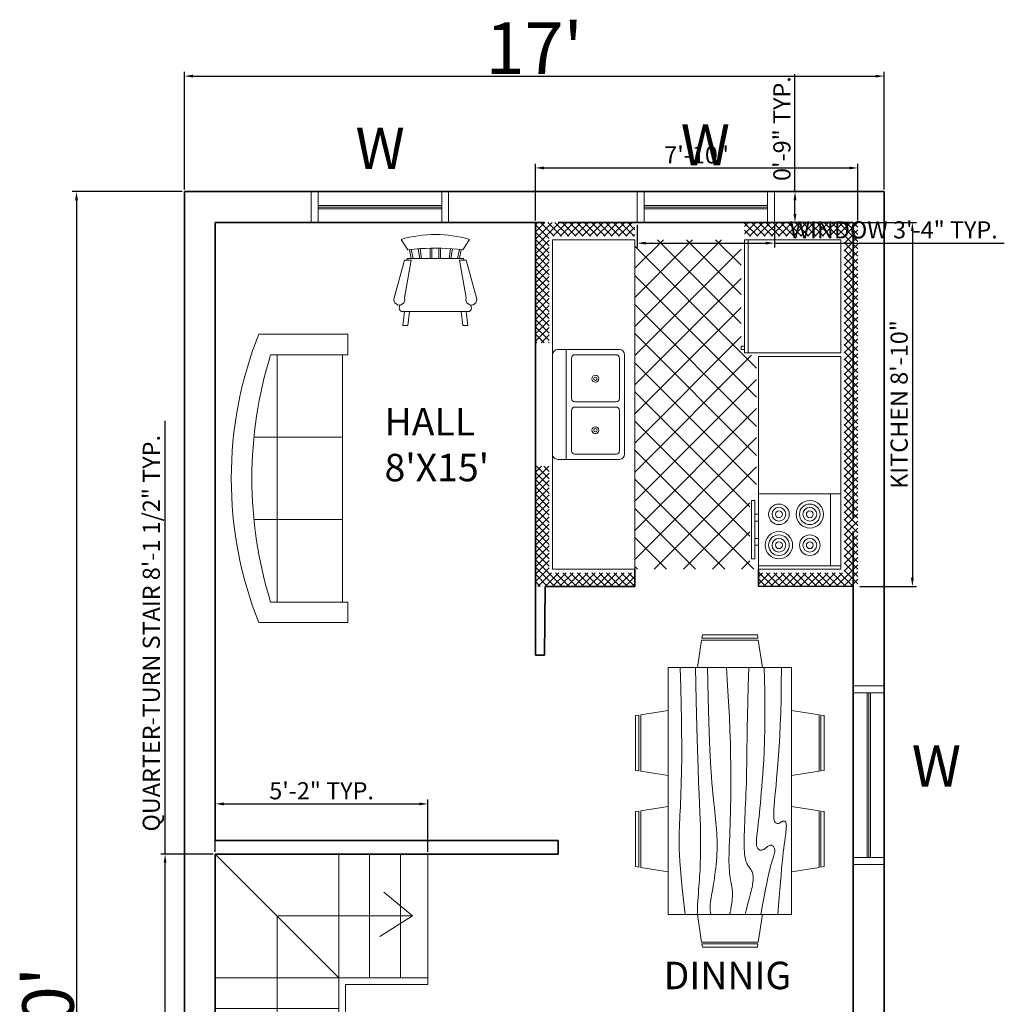
# Model space of a CAD drawing. Units: inches. Extents: x 1662 to 23131, y 1265 to 19127.
# Tile 15 of 26: x 19454 to 19741, y 8502 to 8789. Entities that reach past the tile are written whole.
import ezdxf

# ---------------------------------------------------------------- set-up
doc = ezdxf.new("R2010")
doc.units = ezdxf.units.IN
for name, color, linetype, lineweight in [('A-ANNO-DIMS', 4, 'Continuous', 18), ('A-ANNO-IDEN', 7, 'Continuous', 18), ('A-AREA-IDEN', 7, 'Continuous', 18), ('A-FLOR-CASE', 8, 'Continuous', 18), ('A-FLOR-STRS', 7, 'Continuous', 18), ('A-FURN', 8, 'Continuous', 18), ('A-GLAZ', 4, 'Continuous', 18), ('A-WALL', 7, 'Continuous', 35)]:
    doc.layers.add(name, color=color, linetype=linetype, lineweight=lineweight)
doc.styles.get("Standard").update_dxf_attribs({"font": 'arial.ttf'})
doc.dimstyles.new('ISO-25', dxfattribs={"dimtxt": 5, "dimasz": 2.5, "dimexe": 1.25, "dimexo": 0.625, "dimtad": 1, "dimlunit": 3, "dimtxsty": 'Standard', "dimcen": 2.5, "dimadec": 0, "dimazin": 0, "dimtfac": 1, "dimtmove": 0, "dimatfit": 3, "dimfxl": 1, "dimarcsym": 0})

# ---------------------------------------------------------------- blocks, each defined once
blk = doc.blocks.new('Kitchen Layout - 7 x 8 ft')
for p, q in [((-5, 81.32), (2.68, 89)), ((-5, 83.44), (0.56, 89)), ((-5, 85.56), (-1.56, 89)), ((-5, 87.68), (-3.68, 89)), ((1.09, 85), (-2.91, 89)), ((3.21, 85), (-0.79, 89)), ((0.81, 85), (4.81, 89)), ((5.34, 85), (1.34, 89)), ((2.93, 85), (6.93, 89)), ((7.46, 85), (3.46, 89)), ((5.05, 85), (9.05, 89)), ((9.58, 85), (5.58, 89)), ((7.17, 85), (11.17, 89)), ((11.7, 85), (7.7, 89)), ((9.29, 85), (13.29, 89)), ((13.82, 85), (9.82, 89)), ((11.41, 85), (15.41, 89)), ((15.94, 85), (11.94, 89)), ((13.53, 85), (17.53, 89)), ((18.06, 85), (14.06, 89)), ((15.65, 85), (19.65, 89)), ((20.18, 85), (16.18, 89)), ((17.78, 85), (21.78, 89)), ((22.31, 85), (18.31, 89)), ((19.9, 85), (23.9, 89)), ((24.43, 85), (20.43, 89)), ((22.02, 85), (26.02, 89)), ((26.55, 85), (22.55, 89)), ((24.14, 85), (28.14, 89)), ((28.67, 85), (24.67, 89)), ((26.26, 85), (30.26, 89)), ((30.79, 85), (26.79, 89)), ((28.38, 85), (32.38, 89)), ((32.91, 85), (28.91, 89)), ((30.5, 85), (34.5, 89)), ((35.03, 85), (31.03, 89)), ((32.63, 85), (36.63, 89)), ((37.16, 85), (33.16, 89)), ((34.75, 85), (38.75, 89)), ((39.28, 85), (35.28, 89)), ((36.87, 85), (40.87, 89)), ((41.4, 85), (37.4, 89)), ((38.99, 85), (42.99, 89)), ((43.52, 85), (39.52, 89)), ((41.11, 85), (45.11, 89)), ((45.64, 85), (41.64, 89)), ((43.23, 85), (47.23, 89)), ((47.76, 85), (43.76, 89)), ((45.35, 85), (49.35, 89)), ((49.88, 85), (45.88, 89)), ((47.47, 85), (51.47, 89)), ((52, 85), (48, 89)), ((49.6, 85), (53.6, 89)), ((54.13, 85), (50.13, 89)), ((51.72, 85), (55.72, 89)), ((56.25, 85), (52.25, 89)), ((53.84, 85), (57.84, 89)), ((58.37, 85), (54.37, 89)), ((55.96, 85), (59.96, 89)), ((60.49, 85), (56.49, 89)), ((58.08, 85), (62.08, 89)), ((62.61, 85), (58.61, 89)), ((60.2, 85), (64.2, 89)), ((64.73, 85), (60.73, 89)), ((62.32, 85), (66.32, 89)), ((66.85, 85), (62.85, 89)), ((64.45, 85), (68.45, 89)), ((68.97, 85), (64.97, 89)), ((66.57, 85), (70.57, 89)), ((71.1, 85), (67.1, 89)), ((68.69, 85), (72.69, 89)), ((73.22, 85), (69.22, 89)), ((70.81, 85), (74.81, 89)), ((75.34, 85), (71.34, 89)), ((72.93, 85), (76.93, 89)), ((77.46, 85), (73.46, 89)), ((75.05, 85), (79.05, 89)), ((79.58, 85), (75.58, 89)), ((77.17, 85), (81.17, 89)), ((81.7, 85), (77.7, 89)), ((79.29, 85), (83.29, 89)), ((83.82, 85), (79.82, 89)), ((81.42, 85), (85.42, 89)), ((85.95, 85), (81.95, 89)), ((83.54, 85), (87.54, 89)), ((88.07, 85), (84.07, 89)), ((85.66, 85), (89.66, 89)), ((90.19, 85), (86.19, 89)), ((87.78, 85), (91.78, 89)), ((92.31, 85), (88.31, 89)), ((89.9, 85), (93.9, 89)), ((94.43, 85), (90.43, 89)), ((92.02, 85), (96.02, 89)), ((96.55, 85), (92.55, 89)), ((94.14, 85), (98.14, 89)), ((101, 82.67), (94.67, 89)), ((96.27, 85), (100.27, 89)), ((101, 84.79), (96.79, 89)), ((101, 86.92), (98.92, 89)), ((-1, 84.97), (-5, 88.97)), ((-1, 82.85), (-5, 86.85)), ((97, 83.61), (101, 87.61)), ((-1, 80.73), (-5, 84.73)), ((34, 84), (96, 84)), ((34, 60), (34, 84)), ((96, 84), (96, 60)), ((97, 81.49), (101, 85.49)), ((101, 80.55), (97, 84.55)), ((97, 79.37), (101, 83.37)), ((-5, 79.19), (-1, 83.19)), ((-1, 78.61), (-5, 82.61)), ((-5, 77.07), (-1, 81.07)), ((-1, 76.49), (-5, 80.49)), ((74, 81), (95, 81)), ((101, 78.43), (97, 82.43)), ((97, 77.25), (101, 81.25)), ((-5, 74.95), (-1, 78.95)), ((-1, 74.36), (-5, 78.36)), ((101, 76.31), (97, 80.31)), ((97, 75.13), (101, 79.13)), ((101, 74.19), (97, 78.19)), ((-5, 72.83), (-1, 76.83)), ((-1, 72.24), (-5, 76.24)), ((-5, 70.71), (-1, 74.71)), ((97, 73.01), (101, 77.01)), ((101, 72.07), (97, 76.07)), ((97, 70.89), (101, 74.89)), ((-1, 70.12), (-5, 74.12)), ((-5, 68.59), (-1, 72.59)), ((-1, 68), (-5, 72)), ((101, 69.95), (97, 73.95)), ((97, 68.76), (101, 72.76)), ((101, 67.82), (97, 71.82)), ((-5, 66.47), (-1, 70.47)), ((-1, 65.88), (-5, 69.88)), ((97, 66.64), (101, 70.64)), ((101, 65.7), (97, 69.7)), ((-5, 64.35), (-1, 68.35)), ((-1, 63.76), (-5, 67.76)), ((-5, 62.22), (-1, 66.22)), ((97, 64.52), (101, 68.52)), ((101, 63.58), (97, 67.58)), ((97, 62.4), (101, 66.4)), ((-1, 61.64), (-5, 65.64)), ((-5, 60.1), (-1, 64.1)), ((-1, 59.52), (-5, 63.52)), ((101, 61.46), (97, 65.46)), ((97, 60.28), (101, 64.28)), ((100.34, 60), (97, 63.34)), ((-5, 57.98), (-1, 61.98)), ((-1, 57.39), (-5, 61.39)), ((98.22, 60), (97, 61.22)), ((98.84, 60), (101, 62.16)), ((-1.73, 56), (-5, 59.27)), ((-4.86, 56), (-1, 59.86)), ((-2.74, 56), (-1, 57.74)), ((10.4, 24), (45.9, 59.5)), ((18.88, 24), (54.38, 59.5)), ((27.37, 24), (62.87, 59.5)), ((33.03, 55.11), (37.41, 59.5)), ((67.71, 24), (33.68, 58.04)), ((96, 60), (34, 60)), ((35.85, 24), (71.35, 59.5)), ((76.2, 24), (40.7, 59.5)), ((44.34, 24), (77.84, 57.5)), ((84.68, 24), (49.18, 59.5)), ((52.82, 24), (86.32, 57.5)), ((93.17, 24), (57.67, 59.5)), ((61.31, 24), (96, 58.69)), ((96, 29.65), (66.15, 59.5)), ((96, 38.14), (76.64, 57.5)), ((80, 60), (80, 59)), ((82, 59), (82, 60)), ((96, 46.63), (85.13, 57.5)), ((87, 59), (87, 60)), ((89, 60), (89, 59)), ((96, 55.11), (93.57, 57.54)), ((100.96, 60), (101, 60.04)), ((-3.85, 56), (-5, 57.15)), ((0, 57), (33, 57)), ((0, 30.57), (24.43, 55)), ((0, 39.06), (15.94, 55)), ((0, 47.54), (7.46, 55)), ((1.91, 24), (32.91, 55)), ((33.77, 24), (2.77, 55)), ((42.26, 24), (11.26, 55)), ((50.74, 24), (19.74, 55)), ((59.23, 24), (28.23, 55)), ((31, 55), (31, 56)), ((32, 55), (31, 55)), ((32, 56), (32, 55)), ((25.29, 24), (0, 49.29)), ((69.79, 24), (96, 50.21)), ((16.8, 24), (0, 40.8)), ((78.28, 24), (96, 41.72)), ((8.32, 24), (0, 32.32)), ((86.76, 24), (96, 33.24)), ((-5, 21.92), (-2.92, 24)), ((-5, 19.8), (-1, 23.8)), ((-1, 19.21), (-5, 23.21)), ((-1, 21.33), (-3.67, 24)), ((-1, 23.45), (-1.55, 24)), ((0, 24), (96, 24)), ((0, 0), (0, 24)), ((95.25, 24), (96, 24.75)), ((96, 24), (96, 0)), ((97, 22.1), (98.9, 24)), ((97, 19.97), (101, 23.97)), ((101, 19.03), (97, 23.03)), ((101, 21.16), (98.16, 24)), ((101, 23.28), (100.28, 24)), ((-5, 17.68), (-1, 21.68)), ((-1, 17.09), (-5, 21.09)), ((97, 17.85), (101, 21.85)), ((101, 16.91), (97, 20.91)), ((-5, 15.55), (-1, 19.55)), ((-1, 14.97), (-5, 18.97)), ((-5, 13.43), (-1, 17.43)), ((47.25, 6.5), (47.25, 18.5)), ((48.75, 18.5), (48.75, 6.5)), ((97, 15.73), (101, 19.73)), ((101, 14.79), (97, 18.79)), ((97, 13.61), (101, 17.61)), ((-1, 12.85), (-5, 16.85)), ((-5, 11.31), (-1, 15.31)), ((-1, 10.73), (-5, 14.73)), ((101, 12.67), (97, 16.67)), ((97, 11.49), (101, 15.49)), ((101, 10.55), (97, 14.55)), ((-5, 9.19), (-1, 13.19)), ((-1, 8.6), (-5, 12.6)), ((97, 9.37), (101, 13.37)), ((101, 8.43), (97, 12.43)), ((-5, 7.07), (-1, 11.07)), ((-1, 6.48), (-5, 10.48)), ((-5, 4.95), (-1, 8.95)), ((97, 7.25), (101, 11.25)), ((101, 6.31), (97, 10.31)), ((97, 5.12), (101, 9.12)), ((-1, 4.36), (-5, 8.36)), ((-5, 2.83), (-1, 6.83)), ((-1, 2.24), (-5, 6.24)), ((101, 4.18), (97, 8.18)), ((97, 3), (101, 7)), ((101, 2.06), (97, 6.06)), ((-5, 0.71), (-1, 4.71)), ((-1, 0.12), (-5, 4.12)), ((64, 4), (32, 4)), ((97, 0.88), (101, 4.88)), ((101, -0.06), (97, 3.94)), ((-5, -1.42), (-1, 2.58)), ((2, -5), (-5, 2)), ((-5, -3.54), (-1, 0.46)), ((96, 0), (0, 0)), ((93.24, -5), (101, 2.76)), ((95.36, -5), (101, 0.64)), ((101, -2.18), (97, 1.82)), ((-0.12, -5), (-5, -0.12)), ((-2.25, -5), (-5, -2.25)), ((-4.34, -5), (-0.34, -1)), ((-2.22, -5), (1.78, -1)), ((-0.1, -5), (3.9, -1)), ((4.12, -5), (0.12, -1)), ((2.02, -5), (6.02, -1)), ((6.24, -5), (2.24, -1)), ((4.14, -5), (8.14, -1)), ((8.36, -5), (4.36, -1)), ((6.27, -5), (10.27, -1)), ((10.48, -5), (6.48, -1)), ((8.39, -5), (12.39, -1)), ((12.6, -5), (8.6, -1)), ((10.51, -5), (14.51, -1)), ((14.73, -5), (10.73, -1)), ((12.63, -5), (16.63, -1)), ((16.85, -5), (12.85, -1)), ((14.75, -5), (18.75, -1)), ((18.97, -5), (14.97, -1)), ((16.87, -5), (20.87, -1)), ((21.09, -5), (17.09, -1)), ((18.99, -5), (22.99, -1)), ((23.21, -5), (19.21, -1)), ((21.11, -5), (25.11, -1)), ((25.33, -5), (21.33, -1)), ((23.24, -5), (27.24, -1)), ((27.45, -5), (23.45, -1)), ((25.36, -5), (29.36, -1)), ((29.57, -5), (25.57, -1)), ((27.48, -5), (30, -2.48)), ((30, -3.3), (27.7, -1)), ((30, -1.18), (29.82, -1)), ((66, -2.54), (67.54, -1)), ((66, -4.66), (69.66, -1)), ((69.88, -5), (66, -1.12)), ((67.78, -5), (71.78, -1)), ((72, -5), (68, -1)), ((69.9, -5), (73.9, -1)), ((74.12, -5), (70.12, -1)), ((72.03, -5), (76.03, -1)), ((76.24, -5), (72.24, -1)), ((74.15, -5), (78.15, -1)), ((78.36, -5), (74.36, -1)), ((76.27, -5), (80.27, -1)), ((80.49, -5), (76.49, -1)), ((78.39, -5), (82.39, -1)), ((82.61, -5), (78.61, -1)), ((80.51, -5), (84.51, -1)), ((84.73, -5), (80.73, -1)), ((82.63, -5), (86.63, -1)), ((86.85, -5), (82.85, -1)), ((84.75, -5), (88.75, -1)), ((88.97, -5), (84.97, -1)), ((86.88, -5), (90.88, -1)), ((91.09, -5), (87.09, -1)), ((89, -5), (93, -1)), ((93.21, -5), (89.21, -1)), ((91.12, -5), (95.12, -1)), ((95.34, -5), (91.34, -1)), ((97.46, -5), (93.46, -1)), ((99.58, -5), (95.58, -1)), ((101, -4.3), (97, -0.3)), ((97.48, -5), (101, -1.48)), ((-4.37, -5), (-5, -4.37)), ((29.6, -5), (30, -4.6)), ((67.76, -5), (66, -3.24)), ((99.6, -5), (101, -3.6))]:
    blk.add_line(p, q)
for points in [[(0, 56), (0, 84), (33, 84), (33, 56)], [(74, 60), (74, 84), (95, 84), (95, 60)], [(76, 58), (76, 59), (93, 59), (93, 58)]]:
    blk.add_lwpolyline(points, close=True)
for points in [[(33.5, 21), (62.5, 21)], [(32, 1.5), (32, 19.5)], [(33.5, 6.5), (33.5, 18.5)], [(34.5, 19.5), (46.25, 19.5)], [(49.75, 19.5), (61.5, 19.5)], [(62.5, 18.5), (62.5, 6.5)], [(64, 19.5), (64, 1.5)], [(46.25, 5.5), (34.5, 5.5)], [(61.5, 5.5), (49.75, 5.5)], [(62.5, 0), (33.5, 0)]]:
    blk.add_lwpolyline(points)
for centre, radius in [((80, 75), 4), ((80, 75), 3), ((89, 75), 3), ((80, 75), 2), ((80, 75), 1), ((89, 75), 2), ((89, 75), 1), ((80, 66), 3), ((89, 66), 4), ((89, 66), 3), ((80, 66), 2), ((80, 66), 1), ((89, 66), 2), ((89, 66), 1), ((40.5, 12.5), 1), ((40.5, 12.5), 0.5), ((55.5, 12.5), 1), ((55.5, 12.5), 0.5)]:
    blk.add_circle(centre, radius)
for centre, radius, start, end in [((33.5, 19.5), 1.5, 90, 180), ((62.5, 19.5), 1.5, 0, 90), ((34.5, 18.5), 1, 90, 180), ((46.25, 18.5), 1, 0, 90), ((49.75, 18.5), 1, 90, 180), ((61.5, 18.5), 1, 0, 90), ((34.5, 6.5), 1, 180, 270), ((46.25, 6.5), 1, 270, 0), ((49.75, 6.5), 1, 180, 270), ((61.5, 6.5), 1, 270, 0), ((33.5, 1.5), 1.5, 180, 270), ((62.5, 1.5), 1.5, 270, 0)]:
    blk.add_arc(centre, radius, start, end)
blk = doc.blocks.new('Dining Set - 36 x 72 in.')
for p, q in [((-22.2343, 26.00059), (-23.4847, 17.99762)), ((-22.2304, 26), (-5.7608, 26)), ((-22, 27.5), (-22.1562, 26.50042)), ((-5.8416, 26.5), (-22.1534, 26.5)), ((-22, 27.5), (-6, 27.5)), ((-5.8437, 26.49966), (-6, 27.5)), ((-4.5152, 17.99762), (-5.7655, 25.99926)), ((5.7657, 26.00059), (4.5153, 17.99762)), ((5.7696, 26), (22.2392, 26)), ((6, 27.5), (5.8438, 26.50042)), ((22.1584, 26.5), (5.8466, 26.5)), ((6, 27.5), (22, 27.5)), ((22.1563, 26.49966), (22, 27.5)), ((23.4848, 17.99762), (22.2345, 25.99926)), ((36, 18), (-36, 18)), ((-36, 18), (-36, -18)), ((36, -18), (36, 18)), ((-44.0006, 8.23428), (-35.9976, 9.48474)), ((44.0006, 8.23428), (35.9976, 9.48474)), ((-45.5, 8), (-44.5004, 8.15617)), ((-45.5, 8), (-45.5, -8)), ((-44.5, -8.15843), (-44.5, 8.15338)), ((-44, 8.23041), (-44, -8.23915)), ((44, 8.23041), (44, -8.23915)), ((44.5, -8.15843), (44.5, 8.15338)), ((45.5, 8), (44.5005, 8.15617)), ((45.5, 8), (45.5, -8)), ((-44.4997, -8.15631), (-45.5, -8)), ((-35.9976, -9.48476), (-43.9993, -8.2345)), ((35.9976, -9.48476), (43.9993, -8.2345)), ((44.4997, -8.15631), (45.5, -8)), ((-36, -18), (36, -18)), ((-22.2343, -26.0006), (-23.4847, -17.99762)), ((-4.5152, -17.99762), (-5.7655, -25.99928)), ((5.7657, -26.0006), (4.5153, -17.99762)), ((23.4848, -17.99762), (22.2345, -25.99928)), ((-22.2304, -26), (-5.7608, -26)), ((-22, -27.5), (-22.1562, -26.50044)), ((-5.8416, -26.5), (-22.1534, -26.5)), ((-22, -27.5), (-6, -27.5)), ((-5.8437, -26.49967), (-6, -27.5)), ((5.7696, -26), (22.2392, -26)), ((6, -27.5), (5.8438, -26.50044)), ((22.1584, -26.5), (5.8466, -26.5)), ((6, -27.5), (22, -27.5)), ((22.1563, -26.49967), (22, -27.5))]:
    blk.add_line(p, q)
for points in [[(-36, 15), (-31.1772, 14.97754), (-26.8079, 14.91406), (-22.8538, 14.81543), (-19.276, 14.6875), (-16.0362, 14.53613), (-13.0957, 14.36718), (-10.4159, 14.18652), (-7.9583, 14), (-5.6904, 13.81315), (-3.6035, 13.63021), (-1.6954, 13.45508), (0.0365, 13.29166), (1.5945, 13.14388), (2.9811, 13.01562), (4.1988, 12.9108), (5.25, 12.83333), (6.1393, 12.78613), (6.8802, 12.76823), (7.4883, 12.77767), (7.9792, 12.8125), (8.3685, 12.87077), (8.6719, 12.95052), (8.9049, 13.0498), (9.0833, 13.16666), (9.2205, 13.29899), (9.3216, 13.44401), (9.3895, 13.59879), (9.4271, 13.76041), (9.4373, 13.92594), (9.4232, 14.09245), (9.3875, 14.257), (9.3333, 14.41666), (9.2638, 14.56917), (9.1836, 14.71484), (9.0975, 14.85465), (9.0104, 14.98958), (8.9272, 15.1206), (8.8529, 15.2487), (8.7922, 15.37483), (8.75, 15.5), (8.7305, 15.62467), (8.7344, 15.74739), (8.7617, 15.86621), (8.8125, 15.97916), (8.8867, 16.08431), (8.9844, 16.17968), (9.1055, 16.26334), (9.25, 16.33333), (9.4189, 16.38802), (9.6172, 16.42708), (9.8506, 16.45052), (10.125, 16.45833), (10.4463, 16.45052), (10.8203, 16.42708), (11.2529, 16.38802), (11.75, 16.33333), (12.3184, 16.26318), (12.9694, 16.17838), (13.7151, 16.07991), (14.5677, 15.96875), (15.5395, 15.84586), (16.6426, 15.71224), (17.8893, 15.56884), (19.2917, 15.41666), (20.859, 15.25667), (22.5879, 15.08984), (24.4721, 14.91715), (26.5052, 14.73958), (28.6809, 14.5581), (30.9929, 14.3737), (33.4347, 14.18733), (36, 14)], [(-36, 10), (-28.9766, 10.14274), (-23.1725, 10.20442), (-18.4241, 10.19775), (-14.5677, 10.13541), (-11.4399, 10.03011), (-8.877, 9.89453), (-6.7154, 9.74137), (-4.7917, 9.58333), (-2.9698, 9.43082), (-1.2246, 9.28515), (0.4415, 9.14534), (2.026, 9.01041), (3.5266, 8.87939), (4.9408, 8.7513), (6.266, 8.62516), (7.5, 8.5), (8.6411, 8.37549), (9.6914, 8.2539), (10.6538, 8.13818), (11.5312, 8.03125), (12.3267, 7.93603), (13.043, 7.85547), (13.6831, 7.79248), (14.25, 7.75), (14.7471, 7.7303), (15.1797, 7.73307), (15.5537, 7.75732), (15.875, 7.80208), (16.1494, 7.86637), (16.3828, 7.94922), (16.5811, 8.04964), (16.75, 8.16666), (16.8944, 8.29915), (17.0143, 8.44531), (17.1089, 8.60319), (17.1771, 8.77083), (17.218, 8.94629), (17.2305, 9.1276), (17.2137, 9.31282), (17.1667, 9.5), (17.0895, 9.6875), (16.987, 9.875), (16.8649, 10.0625), (16.7292, 10.25), (16.5856, 10.4375), (16.4401, 10.625), (16.2985, 10.8125), (16.1667, 11), (16.05, 11.18733), (15.9518, 11.3737), (15.8752, 11.5581), (15.8229, 11.73958), (15.798, 11.91715), (15.8034, 12.08984), (15.842, 12.25667), (15.9167, 12.41666), (16.0295, 12.56836), (16.1784, 12.70833), (16.3605, 12.83268), (16.5729, 12.9375), (16.8127, 13.01888), (17.0768, 13.07291), (17.3625, 13.0957), (17.6667, 13.08333), (17.9894, 13.03312), (18.3418, 12.94726), (18.7382, 12.82918), (19.1927, 12.68229), (19.7195, 12.51001), (20.3327, 12.31575), (21.0465, 12.10294), (21.875, 11.875), (22.8357, 11.63354), (23.959, 11.37304), (25.2786, 11.08618), (26.8282, 10.76562), (28.6414, 10.40405), (30.752, 9.99414), (33.1936, 9.52856), (36, 9)], [(-36, 5.5), (-30.7157, 5.3348), (-26.069, 5.20963), (-21.9946, 5.11767), (-18.4271, 5.05208), (-15.3009, 5.00602), (-12.5508, 4.97265), (-10.1112, 4.94515), (-7.9167, 4.91666), (-5.909, 4.88167), (-4.0586, 4.83984), (-2.3429, 4.79215), (-0.7396, 4.73958), (0.7739, 4.6831), (2.22, 4.6237), (3.6213, 4.56233), (5, 4.5), (6.373, 4.43782), (7.7344, 4.3776), (9.0723, 4.32129), (10.375, 4.27083), (11.6309, 4.22819), (12.8281, 4.19531), (13.9551, 4.17415), (15, 4.16666), (15.954, 4.17448), (16.819, 4.19791), (17.6001, 4.23698), (18.3021, 4.29166), (18.9299, 4.36198), (19.4883, 4.44791), (19.9823, 4.54948), (20.4167, 4.66666), (20.7969, 4.79899), (21.1302, 4.94401), (21.4245, 5.09879), (21.6875, 5.26041), (21.9271, 5.42594), (22.1511, 5.59245), (22.3672, 5.757), (22.5834, 5.91666), (22.8065, 6.06868), (23.0404, 6.21093), (23.2879, 6.34147), (23.5521, 6.45833), (23.8358, 6.55957), (24.142, 6.64323), (24.4735, 6.70735), (24.8334, 6.75), (25.2235, 6.76969), (25.642, 6.76692), (26.0858, 6.74267), (26.5521, 6.69791), (27.0379, 6.63362), (27.5404, 6.55078), (28.0565, 6.45036), (28.5834, 6.33333), (29.1242, 6.19987), (29.7071, 6.04687), (30.3661, 5.87044), (31.1354, 5.66666), (32.0493, 5.43164), (33.142, 5.16146), (34.4475, 4.85221), (36, 4.5)], [(-36, -1), (-30.7915, -0.6591), (-26.0195, -0.38216), (-21.6519, -0.16284), (-17.6563, 0.00521), (-14.0005, 0.12833), (-10.6523, 0.21289), (-7.5796, 0.26522), (-4.75, 0.29166), (-2.134, 0.29793), (0.2878, 0.28711), (2.5317, 0.26163), (4.6146, 0.22396), (6.5529, 0.17651), (8.3633, 0.12174), (10.0623, 0.06209), (11.6667, 0), (13.1899, -0.06201), (14.6341, -0.1211), (15.9982, -0.17432), (17.2813, -0.21875), (18.4823, -0.25147), (19.6003, -0.26953), (20.6343, -0.27002), (21.5834, -0.25), (22.4481, -0.20768), (23.2357, -0.14584), (23.9549, -0.06836), (24.6146, 0.02083), (25.2235, 0.11784), (25.7904, 0.21875), (26.3241, 0.31966), (26.8334, 0.41666), (27.3265, 0.50618), (27.8099, 0.58593), (28.2894, 0.65397), (28.7709, 0.70833), (29.2601, 0.74707), (29.763, 0.76823), (30.2855, 0.76985), (30.8334, 0.75), (31.4088, 0.70784), (31.9994, 0.64713), (32.589, 0.57275), (33.1615, 0.48958), (33.7008, 0.4025), (34.1908, 0.3164), (34.6153, 0.23616), (34.9584, 0.16666), (35.2099, 0.11165), (35.3848, 0.07031), (35.504, 0.04069), (35.5886, 0.02083), (35.6594, 0.00879), (35.7377, 0.0026), (35.8442, 0.00032), (36, 0)], [(-36, -6.5), (-27.1843, -6.31267), (-20.084, -6.1263), (-14.469, -5.9419), (-10.1094, -5.76042), (-6.7752, -5.58285), (-4.2363, -5.41016), (-2.2629, -5.24333), (-0.625, -5.08334), (0.8708, -4.93099), (2.2715, -4.78646), (3.5872, -4.64974), (4.8281, -4.52084), (6.0046, -4.39974), (7.127, -4.28646), (8.2053, -4.18099), (9.25, -4.08334), (10.2705, -3.99382), (11.2734, -3.91407), (12.2647, -3.84603), (13.25, -3.79167), (14.2354, -3.75293), (15.2266, -3.73177), (16.2295, -3.73015), (17.25, -3.75), (18.2912, -3.79248), (19.3451, -3.85547), (20.4009, -3.93604), (21.4479, -4.03125), (22.4754, -4.13819), (23.4727, -4.25391), (24.4289, -4.37549), (25.3334, -4.5), (26.1785, -4.62492), (26.9694, -4.74935), (27.7145, -4.87281), (28.4219, -4.99479), (29.1, -5.11483), (29.7572, -5.23242), (30.4016, -5.34709), (31.0417, -5.45834), (31.6837, -5.56437), (32.3262, -5.65821), (32.9658, -5.73153), (33.599, -5.77604), (34.2224, -5.78345), (34.8327, -5.74545), (35.4264, -5.65373), (36, -5.5)], [(-36, -10), (-26.4022, -9.81299), (-18.4675, -9.62891), (-11.9839, -9.45069), (-6.7396, -9.28125), (-2.5226, -9.12354), (0.8789, -8.98047), (3.6769, -8.85498), (6.0833, -8.75), (8.2767, -8.66765), (10.3021, -8.60677), (12.1712, -8.56543), (13.8958, -8.54167), (15.4876, -8.53353), (16.9583, -8.53907), (18.3197, -8.55632), (19.5834, -8.58334), (20.7616, -8.61841), (21.8685, -8.66081), (22.9188, -8.71004), (23.9271, -8.76563), (24.9081, -8.82707), (25.8763, -8.89388), (26.8465, -8.96558), (27.8334, -9.04167), (28.8474, -9.12118), (29.8828, -9.20117), (30.93, -9.27824), (31.9792, -9.34896), (33.0205, -9.40991), (34.0443, -9.45768), (35.0407, -9.48885), (36, -9.5)], [(-36, -14.5), (-30.0881, -14.33513), (-25.0332, -14.21224), (-20.7312, -14.12647), (-17.0781, -14.07292), (-13.97, -14.04671), (-11.3027, -14.04297), (-8.9724, -14.05681), (-6.875, -14.08334), (-4.9224, -14.11833), (-3.0905, -14.16016), (-1.3709, -14.20785), (0.2448, -14.26042), (1.7647, -14.3169), (3.1973, -14.3763), (4.5507, -14.43767), (5.8333, -14.5), (7.0554, -14.5621), (8.235, -14.62175), (9.3922, -14.67652), (10.5469, -14.72396), (11.7192, -14.76164), (12.929, -14.78711), (14.1965, -14.79794), (15.5417, -14.79167), (16.9933, -14.76424), (18.6152, -14.70508), (20.4804, -14.60197), (22.6615, -14.44271), (25.2312, -14.21509), (28.2624, -13.9069), (31.8277, -13.50594), (36, -13)]]:
    blk.add_lwpolyline(points)
blk = doc.blocks.new('Sofa - Roundback 7 ft.')
for p, q in [((-12.00002, -32.4421), (-12.00003, -6.5971)), ((11.99997, -32.4421), (11.99998, -6.5971)), ((-36.000027, -34), (-36.000027, -11.4696)), ((35.99998, -34), (35.99998, -11.4696)), ((-35.999844, -13.3819), (35.9998, -13.3819)), ((-36.000027, -32.4421), (35.99998, -32.4421))]:
    blk.add_line(p, q)
for points in [[(-36.000027, -34), (-42.000027, -34), (-42.000027, -8)], [(41.99998, -8), (41.99998, -34), (35.99998, -34)]]:
    blk.add_lwpolyline(points)
for centre, radius, start, end in [((0, -114.25), 114.25, 68.43141, 111.5686), ((-0.00001, -127.1968), 121.1968, 72.72033, 107.2797)]:
    blk.add_arc(centre, radius, start, end)
blk = doc.blocks.new('Chair - Rocking')
for p, q in [((-8, -4.5), (-10, -1.5)), ((8, -4.5), (10, -1.5)), ((-7.5, -4.5), (-7, -7)), ((-6.5, -7), (-7.02225, -4.43)), ((-4.5, -7), (-4.96674, -4.19951)), ((-4, -7), (-4.40532, -4.16272)), ((-1.5, -4.05012), (-1.5, -7)), ((-1, -7), (-1, -4.05012)), ((1, -7), (1, -4.04655)), ((1.5, -4.05012), (1.5, -7)), ((4, -7), (4.40187, -4.18694)), ((4.5, -7), (4.96761, -4.19437)), ((6.5, -7), (7, -4.4057)), ((7.5, -4.5), (7, -7)), ((-9, -7.5), (-12, -18.49999)), ((-7, -7.5), (-9, -7.5)), ((-9, -18.49999), (-7, -7.5)), ((-8.23428, -6.99939), (-8.3093, -7.47958)), ((-8.23041, -7), (8.23915, -7)), ((7, -7.5), (9, -7.5)), ((9, -18.49999), (7, -7.5)), ((8.31071, -7.48854), (8.23449, -7.00073)), ((9, -7.5), (12, -18.49999)), ((-10.36644, -20.64523), (-10.5, -21.49999)), ((-9, -22.49999), (-9.5, -26.49999)), ((0, -22.49999), (-9.5, -22.49999)), ((-8, -26.49999), (-7.5, -22.49999)), ((0, -22.49999), (9.5, -22.49999)), ((8, -26.49999), (7.5, -22.49999)), ((9, -22.49999), (9.5, -26.49999)), ((10.5, -21.49999), (10.3575, -20.58798)), ((-9.5, -26.49999), (-8, -26.49999)), ((9.5, -26.49999), (8, -26.49999))]:
    blk.add_line(p, q)
for centre, radius, start, end in [((0, -34.08333), 34.08333, 72.93847, 107.0615), ((0, -68.25004), 64.25, 93.92211, 97.15267), ((0, -68.25004), 64.25, 82.84733, 93.92211), ((-10.5, -18.99999), 1.58114, 161.5651, 18.43495), ((10.5, -18.99999), 1.58114, 161.5651, 18.43495), ((-9.5, -21.49999), 1, 180, 270), ((9.5, -21.49999), 1, 270, 0)]:
    blk.add_arc(centre, radius, start, end)
blk = doc.blocks.new('*D94')
at = {"layer": 'A-ANNO-DIMS', "color": 0, "lineweight": -2, "transparency": 16777216}
for p, q in [((19502.16, 8739.35), (19502.16, 8773.63)), ((19504.66, 8772.38), (19703.66, 8772.38)), ((19706.16, 8739.35), (19706.16, 8773.63))]:
    blk.add_line(p, q, dxfattribs=at)
at = {"layer": 'A-ANNO-DIMS', "color": 0, "transparency": 16777216}
for points in [[(19504.66, 8772.79), (19504.66, 8771.96), (19502.16, 8772.38)], [(19703.66, 8772.79), (19703.66, 8771.96), (19706.16, 8772.38)]]:
    blk.add_solid(points, dxfattribs=at)
at = {"layer": 'Defpoints', "color": 0, "transparency": 16777216}
for p in [(19706.16, 8772.38), (19502.16, 8738.72), (19706.16, 8738.72)]:
    blk.add_point(p, dxfattribs=at)
at = {"layer": 'A-ANNO-DIMS', "color": 0, "transparency": 16777216, "insert": (19604.16, 8780.53), "char_height": 5, "attachment_point": 5}
blk.add_mtext("{\\H3x;17'}", dxfattribs=at)
blk = doc.blocks.new('*D95')
at = {"layer": 'A-ANNO-DIMS', "color": 0, "lineweight": -2, "transparency": 16777216}
for p, q in [((19501.54, 8738.72), (19469.46, 8738.72)), ((19470.71, 8736.22), (19470.71, 8261.22)), ((19501.54, 8258.72), (19469.46, 8258.72))]:
    blk.add_line(p, q, dxfattribs=at)
at = {"layer": 'A-ANNO-DIMS', "color": 0, "transparency": 16777216}
for points in [[(19470.29, 8736.22), (19471.12, 8736.22), (19470.71, 8738.72)], [(19470.29, 8261.22), (19471.12, 8261.22), (19470.71, 8258.72)]]:
    blk.add_solid(points, dxfattribs=at)
at = {"layer": 'Defpoints', "color": 0, "transparency": 16777216}
for p in [(19502.16, 8738.72), (19470.71, 8258.72), (19502.16, 8258.72)]:
    blk.add_point(p, dxfattribs=at)
at = {"layer": 'A-ANNO-DIMS', "color": 0, "transparency": 16777216, "insert": (19462.42, 8498.72), "char_height": 5, "attachment_point": 5, "rotation": 90}
blk.add_mtext("{\\H3x;40'}", dxfattribs=at)
blk = doc.blocks.new('WIN-48-J9X2')
for p, q in [((9, 52), (0, 52)), ((9, 50), (0, 50)), ((4, 50), (4, 2)), ((4.5, 50), (4.5, 2)), ((5, 50), (5, 2)), ((9, 2), (0, 2)), ((9, 0), (0, 0))]:
    blk.add_line(p, q)
blk = doc.blocks.new('WIN-36-J9X2')
for p, q in [((0, 0), (0, 9)), ((2, 0), (2, 9)), ((38, 0), (38, 9)), ((40, 0), (40, 9)), ((38, 5), (2, 5)), ((38, 4.5), (2, 4.5)), ((38, 4), (2, 4))]:
    blk.add_line(p, q)
blk = doc.blocks.new('STAIR-QUARTER-TURN')
for p, q in [((36, 61.57), (0, 97.57)), ((36, 61.57), (36, 97.57)), ((45, 61.57), (45, 97.57)), ((54, 61.57), (54, 97.57)), ((62, 59.57), (62, 97.57)), ((57.46, 79.57), (49.14, 86.54)), ((18, 79.57), (18, 0)), ((18, 79.57), (57.46, 79.57)), ((57.46, 79.57), (47.96, 73.62)), ((36, 61.57), (0, 61.57)), ((36, 7.57), (36, 61.57)), ((36, 61.57), (62, 61.57)), ((38, 7.57), (38, 59.57)), ((38, 59.57), (62, 59.57)), ((36, 52.57), (0, 52.57)), ((36, 43.57), (0, 43.57)), ((36, 34.57), (0, 34.57)), ((36, 25.57), (0, 25.57)), ((36, 16.57), (0, 16.57)), ((38, 7.57), (0, 7.57))]:
    blk.add_line(p, q)
blk = doc.blocks.new('*D163')
at = {"layer": 'A-ANNO-DIMS', "color": 0, "lineweight": -2, "transparency": 16777216}
for p, q in [((19634.16, 8729.1), (19634.16, 8722.47)), ((19674.16, 8729.1), (19674.16, 8722.47)), ((19636.66, 8723.72), (19671.66, 8723.72)), ((19674.16, 8723.72), (19741.18, 8723.72))]:
    blk.add_line(p, q, dxfattribs=at)
at = {"layer": 'A-ANNO-DIMS', "color": 0, "transparency": 16777216}
for points in [[(19636.66, 8724.14), (19636.66, 8723.31), (19634.16, 8723.72)], [(19671.66, 8724.14), (19671.66, 8723.31), (19674.16, 8723.72)]]:
    blk.add_solid(points, dxfattribs=at)
at = {"layer": 'Defpoints', "color": 0, "transparency": 16777216}
for p in [(19634.16, 8729.72), (19674.16, 8729.72), (19674.16, 8723.72)]:
    blk.add_point(p, dxfattribs=at)
at = {"layer": 'A-ANNO-DIMS', "color": 0, "transparency": 16777216, "insert": (19708.92, 8726.94), "char_height": 5, "attachment_point": 5}
blk.add_mtext('WINDOW 3\'-4" TYP.', dxfattribs=at)
blk = doc.blocks.new('*D164')
at = {"layer": 'A-ANNO-DIMS', "color": 0, "lineweight": -2, "transparency": 16777216}
for p, q in [((19680.16, 8738.72), (19680.16, 8772.95)), ((19674.79, 8738.72), (19681.41, 8738.72)), ((19680.16, 8732.22), (19680.16, 8736.22)), ((19674.79, 8729.72), (19681.41, 8729.72))]:
    blk.add_line(p, q, dxfattribs=at)
at = {"layer": 'A-ANNO-DIMS', "color": 0, "transparency": 16777216}
for points in [[(19679.75, 8736.22), (19680.58, 8736.22), (19680.16, 8738.72)], [(19679.75, 8732.22), (19680.58, 8732.22), (19680.16, 8729.72)]]:
    blk.add_solid(points, dxfattribs=at)
at = {"layer": 'Defpoints', "color": 0, "transparency": 16777216}
for p in [(19674.16, 8738.72), (19680.16, 8738.72), (19674.16, 8729.72)]:
    blk.add_point(p, dxfattribs=at)
at = {"layer": 'A-ANNO-DIMS', "color": 0, "transparency": 16777216, "insert": (19676.99, 8757.09), "char_height": 5, "attachment_point": 5, "rotation": 90}
blk.add_mtext('0\'-9" TYP.', dxfattribs=at)
blk = doc.blocks.new('*D193')
at = {"layer": 'A-ANNO-DIMS', "color": 0, "lineweight": -2, "transparency": 16777216}
for p, q in [((19496.53, 8545.72), (19496.53, 8671.92)), ((19510.54, 8545.72), (19495.28, 8545.72)), ((19496.53, 8450.65), (19496.53, 8543.22)), ((19510.54, 8448.15), (19495.28, 8448.15))]:
    blk.add_line(p, q, dxfattribs=at)
at = {"layer": 'A-ANNO-DIMS', "color": 0, "transparency": 16777216}
for points in [[(19496.11, 8543.22), (19496.94, 8543.22), (19496.53, 8545.72)], [(19496.11, 8450.65), (19496.94, 8450.65), (19496.53, 8448.15)]]:
    blk.add_solid(points, dxfattribs=at)
at = {"layer": 'Defpoints', "color": 0, "transparency": 16777216}
for p in [(19496.53, 8545.72), (19511.16, 8545.72), (19511.16, 8448.15)]:
    blk.add_point(p, dxfattribs=at)
at = {"layer": 'A-ANNO-DIMS', "color": 0, "transparency": 16777216, "insert": (19493.16, 8610.07), "char_height": 5, "attachment_point": 5, "rotation": 90}
blk.add_mtext('QUARTER-TURN STAIR 8\'-1 1/2" TYP.', dxfattribs=at)
blk = doc.blocks.new('*D194')
at = {"layer": 'A-ANNO-DIMS', "color": 0, "lineweight": -2, "transparency": 16777216}
for p, q in [((19511.16, 8546.35), (19511.16, 8561.61)), ((19513.66, 8560.36), (19570.66, 8560.36)), ((19573.16, 8546.35), (19573.16, 8561.61))]:
    blk.add_line(p, q, dxfattribs=at)
at = {"layer": 'A-ANNO-DIMS', "color": 0, "transparency": 16777216}
for points in [[(19513.66, 8560.77), (19513.66, 8559.94), (19511.16, 8560.36)], [(19570.66, 8560.77), (19570.66, 8559.94), (19573.16, 8560.36)]]:
    blk.add_solid(points, dxfattribs=at)
at = {"layer": 'Defpoints', "color": 0, "transparency": 16777216}
for p in [(19573.16, 8560.36), (19511.16, 8545.72), (19573.16, 8545.72)]:
    blk.add_point(p, dxfattribs=at)
at = {"layer": 'A-ANNO-DIMS', "color": 0, "transparency": 16777216, "insert": (19542.16, 8563.54), "char_height": 5, "attachment_point": 5}
blk.add_mtext('5\'-2" TYP.', dxfattribs=at)
blk = doc.blocks.new('*D197')
at = {"layer": 'A-ANNO-DIMS', "color": 0, "lineweight": -2, "transparency": 16777216}
for p, q in [((19699.11, 8729.72), (19715.63, 8729.72)), ((19714.38, 8727.22), (19714.38, 8626.22)), ((19699.11, 8623.72), (19715.63, 8623.72))]:
    blk.add_line(p, q, dxfattribs=at)
at = {"layer": 'A-ANNO-DIMS', "color": 0, "transparency": 16777216}
for points in [[(19713.97, 8727.22), (19714.8, 8727.22), (19714.38, 8729.72)], [(19713.97, 8626.22), (19714.8, 8626.22), (19714.38, 8623.72)]]:
    blk.add_solid(points, dxfattribs=at)
at = {"layer": 'Defpoints', "color": 0, "transparency": 16777216}
for p in [(19698.48, 8729.72), (19698.48, 8623.72), (19714.38, 8623.72)]:
    blk.add_point(p, dxfattribs=at)
at = {"layer": 'A-ANNO-DIMS', "color": 0, "transparency": 16777216, "insert": (19711.17, 8676.72), "char_height": 5, "attachment_point": 5, "rotation": 90}
blk.add_mtext('KITCHEN 8\'-10"', dxfattribs=at)
blk = doc.blocks.new('*D198')
at = {"layer": 'A-ANNO-DIMS', "color": 0, "lineweight": -2, "transparency": 16777216}
for p, q in [((19604.48, 8730.35), (19604.48, 8746.87)), ((19698.48, 8730.35), (19698.48, 8746.87)), ((19606.98, 8745.62), (19695.98, 8745.62))]:
    blk.add_line(p, q, dxfattribs=at)
at = {"layer": 'A-ANNO-DIMS', "color": 0, "transparency": 16777216}
for points in [[(19606.98, 8746.04), (19606.98, 8745.21), (19604.48, 8745.62)], [(19695.98, 8746.04), (19695.98, 8745.21), (19698.48, 8745.62)]]:
    blk.add_solid(points, dxfattribs=at)
at = {"layer": 'Defpoints', "color": 0, "transparency": 16777216}
for p in [(19698.48, 8745.62), (19604.48, 8729.72), (19698.48, 8729.72)]:
    blk.add_point(p, dxfattribs=at)
at = {"layer": 'A-ANNO-DIMS', "color": 0, "transparency": 16777216, "insert": (19651.48, 8748.8), "char_height": 5, "attachment_point": 5}
blk.add_mtext('7\'-10"', dxfattribs=at)

msp = doc.modelspace()

# ---------------------------------------------------------------- linework, layer by layer
at = {"layer": 'A-WALL'}
for p, q in [((19502.163, 8738.722), (19706.163, 8738.722)), ((19502.163, 8258.722), (19502.163, 8738.722)), ((19706.163, 8738.722), (19706.163, 8282.722)), ((19511.163, 8729.722), (19607.163, 8729.722)), ((19511.163, 8549.722), (19511.163, 8729.722)), ((19604.484, 8729.722), (19604.484, 8603.722)), ((19611.163, 8729.722), (19697.163, 8729.722)), ((19697.163, 8729.722), (19697.163, 8643.722)), ((19697.163, 8639.722), (19697.163, 8497.722)), ((19633.458, 8623.722), (19633.484, 8628.722)), ((19669.484, 8628.722), (19669.484, 8623.758)), ((19607.163, 8603.722), (19607.304, 8623.722)), ((19607.304, 8623.722), (19633.458, 8623.722)), ((19669.484, 8623.758), (19697.097, 8623.722)), ((19604.484, 8603.722), (19607.163, 8603.722)), ((19511.163, 8549.722), (19611.163, 8549.722)), ((19611.163, 8545.722), (19611.163, 8549.722)), ((19511.163, 8545.722), (19611.163, 8545.722)), ((19511.163, 8377.722), (19511.163, 8545.722))]:
    msp.add_line(p, q, dxfattribs=at)

# ---------------------------------------------------------------- block references
at = {"layer": 'A-FLOR-CASE', "rotation": 270}
msp.add_blockref('Kitchen Layout - 7 x 8 ft', (19609.484, 8724.722), dxfattribs=at)
at = {"layer": 'A-FLOR-STRS'}
msp.add_blockref('STAIR-QUARTER-TURN', (19511.163, 8448.15), dxfattribs=at)
at = {"layer": 'A-FURN'}
msp.add_blockref('Chair - Rocking', (19575.316, 8726.269), dxfattribs=at)
for name, p, rotation in [('Sofa - Roundback 7 ft.', (19515.827, 8655.173), 89.99999999999999), ('Dining Set - 36 x 72 in.', (19661.187, 8564.101), 270)]:
    msp.add_blockref(name, p, dxfattribs=dict(at, rotation=rotation))
at = {"layer": 'A-GLAZ'}
for name, p in [('WIN-36-J9X2', (19539.163, 8729.722)), ('WIN-36-J9X2', (19634.163, 8729.722)), ('WIN-48-J9X2', (19697.163, 8542.722))]:
    msp.add_blockref(name, p, dxfattribs=at)

# ---------------------------------------------------------------- texts
at = {"layer": 'A-ANNO-IDEN', "char_height": 12, "attachment_point": 1}
for insert in [(19646.85, 8758.346), (19552.04, 8757.338), (19714.2, 8577.423)]:
    msp.add_mtext_dynamic_manual_height_columns('W', width=471.52273, gutter_width=12.5, heights=[28.462], dxfattribs=dict(at, insert=insert))
at = {"layer": 'A-AREA-IDEN', "char_height": 8, "attachment_point": 1}
for s, insert in [("HALL \\P8'X15'", (19560.499, 8675.684)), (' DINNIG', (19639.42, 8514.382))]:
    msp.add_mtext_dynamic_manual_height_columns(s, width=1142.59551, gutter_width=12.5, heights=[277.772], dxfattribs=dict(at, insert=insert))

# ---------------------------------------------------------------- dimensions: what is measured, and where the dimension line sits
at = {"layer": 'A-ANNO-DIMS'}
for base, p1, p2, text, override, picture, middle in [((19706.163, 8772.377), (19502.163, 8738.722), (19706.163, 8738.722), '{\\H3x;<>}', {"dimclrd": 0, "dimclre": 0, "dimclrt": 0}, '*D94', (19604.163, 8780.532)), ((19674.163, 8723.722), (19634.163, 8729.722), (19674.163, 8729.722), 'WINDOW <> TYP.', {"dimdec": 1, "dimlfac": 1, "dimrnd": 0, "dimzin": 1, "dimdsep": 46, "dimlunit": 4, "dimfrac": 2}, '*D163', (19708.924, 8726.936)), ((19573.163, 8560.358), (19511.163, 8545.722), (19573.163, 8545.722), '<> TYP.', {"dimdec": 1, "dimlfac": 1, "dimrnd": 0, "dimzin": 1, "dimdsep": 46, "dimlunit": 4, "dimfrac": 2}, '*D194', (19542.163, 8563.536))]:
    dim = msp.add_linear_dim(base=base, p1=p1, p2=p2, text=text, dimstyle='ISO-25', override=override, dxfattribs=at)
    dim.commit()
    dim.dimension.update_dxf_attribs({"geometry": picture, "text_midpoint": middle})
for base, p1, p2, angle, text, override, picture, middle in [((19680.163, 8738.722), (19674.163, 8729.722), (19674.163, 8738.722), 90, '<> TYP.', {"dimdec": 1, "dimlfac": 1, "dimrnd": 0, "dimzin": 1, "dimdsep": 46, "dimlunit": 4, "dimfrac": 2}, '*D164', (19676.985, 8757.086)), ((19470.707, 8258.722), (19502.163, 8738.722), (19502.163, 8258.722), 90, '{\\H3x;<>}', {"dimclrd": 0, "dimclre": 0, "dimclrt": 0}, '*D95', (19462.424, 8498.722)), ((19714.384, 8623.722), (19698.484, 8729.722), (19698.484, 8623.722), 270, 'KITCHEN <>', {"dimdec": 1, "dimlfac": 1, "dimrnd": 0, "dimzin": 1, "dimdsep": 46, "dimlunit": 4, "dimfrac": 2}, '*D197', (19711.173, 8676.722)), ((19496.528, 8545.722), (19511.163, 8448.15), (19511.163, 8545.722), 90, 'QUARTER-TURN STAIR <> TYP.', {"dimdec": 1, "dimlfac": 1, "dimrnd": 0, "dimzin": 1, "dimdsep": 46, "dimlunit": 4, "dimfrac": 2}, '*D193', (19493.164, 8610.07))]:
    dim = msp.add_linear_dim(base=base, p1=p1, p2=p2, angle=angle, text=text, dimstyle='ISO-25', override=override, dxfattribs=at)
    dim.commit()
    dim.dimension.update_dxf_attribs({"geometry": picture, "text_midpoint": middle})
dim = msp.add_linear_dim(base=(19698.484, 8745.622), p1=(19604.484, 8729.722), p2=(19698.484, 8729.722), dimstyle='ISO-25', override={"dimdec": 1, "dimlfac": 1, "dimrnd": 0, "dimzin": 1, "dimdsep": 46, "dimlunit": 4, "dimfrac": 2}, dxfattribs=at)
dim.commit()
dim.dimension.update_dxf_attribs({"geometry": '*D198', "text_midpoint": (19651.484, 8748.8)})

doc.saveas('drawing.dxf')
